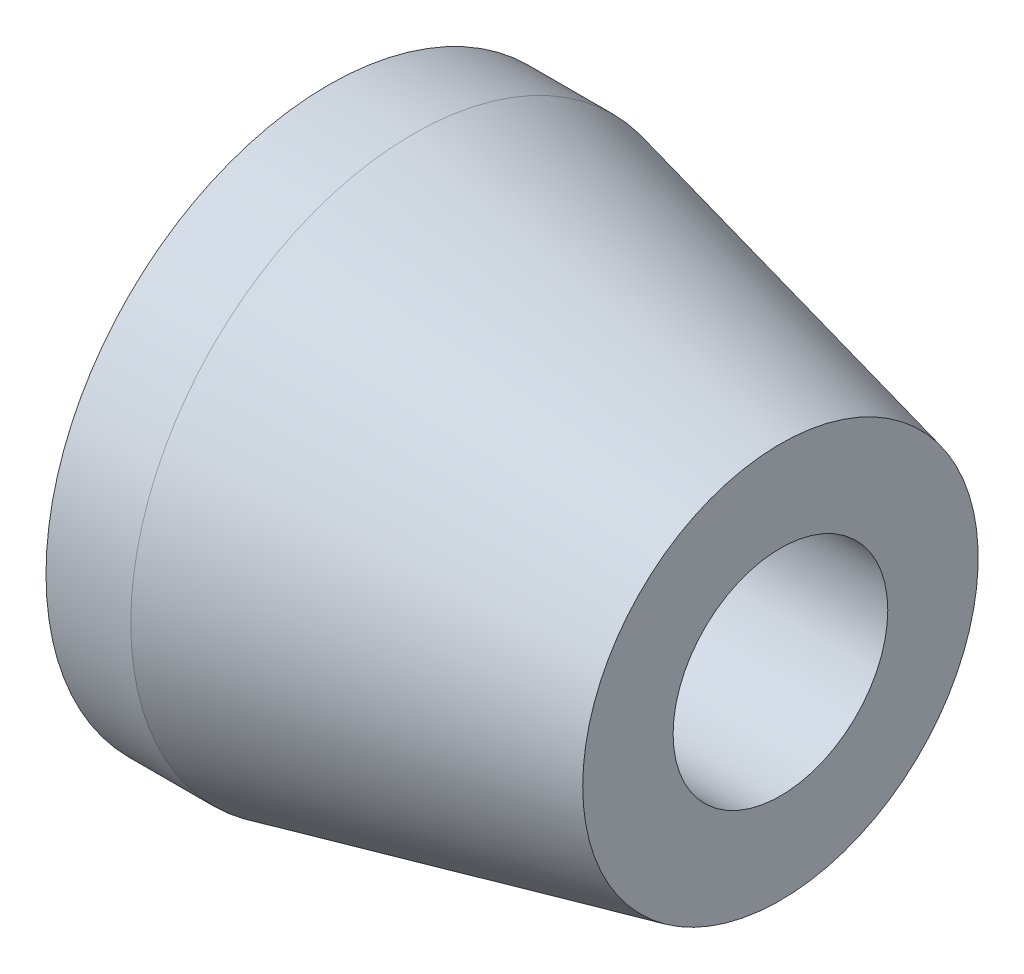
SolidWorks part; units mm, degrees
material "Plain Carbon Steel"
ref_plane "Front Plane" through (0, 0, 0) normal (0, 0, 1) x (1, 0, 0)
ref_plane "Top Plane" through (0, 0, 0) normal (0, 1, 0) x (1, 0, 0)
ref_plane "Right Plane" through (0, 0, 0) normal (1, 0, 0) x (0, 0, -1)
sketch "Bush Profile Sketch" plane through (0, 0, 0) normal (0, 0, 1) x (1, 0, 0)
  line L0 (-1000, 0) -> (49000, 0) construction
  line L1 (0, -1000) -> (0, 49000) construction
  line L7 (0, 0) -> (0, 10)
  line L8 (0, 10) -> (3, 10)
  line L9 (3, 10) -> (16, 7)
  line L10 (16, 7) -> (16, 0)
  line L11 (16, 0) -> (0, 0)
  dimension "D1" = 3
  dimension "D2" = 16
  dimension "D3" = 7
  dimension "D4" = 10
revolve "Bush Body" add sketch "Bush Profile Sketch" angle 360 about L0
sketch "Bore Sketch" plane through (0, 0, 0) normal (-1, 0, 0) x (0, 0, 1)
  line L0 (-1000, 0) -> (49000, 0) construction
  line L1 (0, -1000) -> (0, 49000) construction
  circle A0 centre (0, 0) radius 3.8
  dimension "D1" = 7.6
extrude "Through Bore" cut sketch "Bore Sketch" against normal through all
sketch "Recess Sketch Ø13" plane through (0, 0, 0) normal (-1, 0, 0) x (0, 0, 1)
  circle A0 centre (0, 0) radius 6.5
  dimension "D1" = 13
extrude "Recess Ø13x2" cut sketch "Recess Sketch Ø13" against normal blind 2
